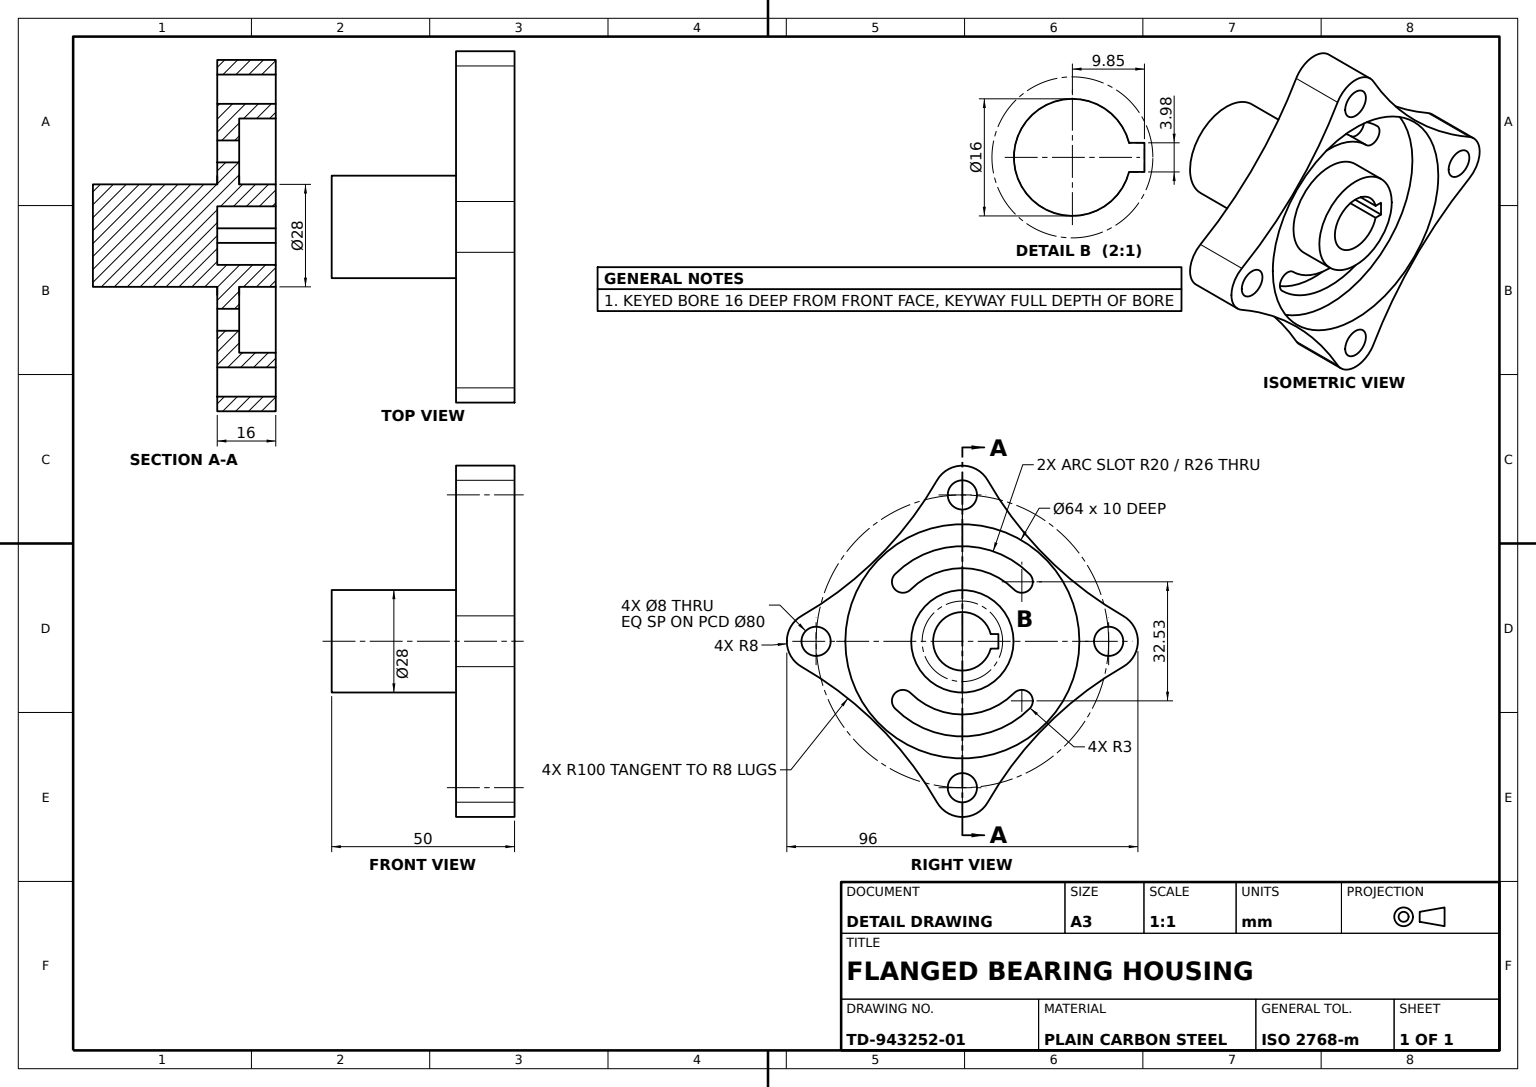
SolidWorks part; units mm, degrees
material "Plain Carbon Steel"
ref_plane "Front Plane" through (0, 0, 0) normal (0, 0, 1) x (1, 0, 0)
ref_plane "Top Plane" through (0, 0, 0) normal (0, 1, 0) x (1, 0, 0)
ref_plane "Right Plane" through (0, 0, 0) normal (1, 0, 0) x (0, 0, -1)
sketch "Flange Plate Sketch" plane through (0, 0, 0) normal (0, 0, 1) x (1, 0, 0)
  line L0 (0, 0) -> (0, 40) construction
  line L1 (0, 0) -> (40, 0) construction
  line L2 (0, 0) -> (0, -40) construction
  line L3 (0, 0) -> (-40, 0) construction
  circle A0 centre (0, 0) radius 40 construction
  circle A1 centre (0, 0) radius 32
  circle A2 centre (0, 40) radius 4
  circle A4 centre (40, 0) radius 4
  circle A5 centre (-40, 0) radius 4
  circle A6 centre (0, -40) radius 4
  arc A7 (6.9409, 43.9779) -> (-6.9409, 43.9779) centre (0, 40) ccw
  arc A8 (-43.9779, 6.9409) -> (-43.9779, -6.9409) centre (-40, 0) ccw
  arc A9 (-6.9409, -43.9779) -> (6.9409, -43.9779) centre (0, -40) ccw
  arc A10 (43.9779, -6.9409) -> (43.9779, 6.9409) centre (40, 0) ccw
  arc A11 (-43.9779, 6.9409) -> (-6.9409, 43.9779) centre (-93.7021, 93.7021) ccw
  arc A12 (6.9409, 43.9779) -> (43.9779, 6.9409) centre (93.7021, 93.7021) ccw
  arc A13 (6.9409, 43.9779) -> (43.9779, 6.9409) centre (93.7021, 93.7021) ccw
  arc A14 (43.9779, -6.9409) -> (6.9409, -43.9779) centre (93.7021, -93.7021) ccw
  arc A15 (-6.9409, -43.9779) -> (-43.9779, -6.9409) centre (-93.7021, -93.7021) ccw
  dimension "D1" = 40
  dimension "D2" = 32
  dimension "D3" = 4
  dimension "D4" = 4
  dimension "D5" = 4
  dimension "D6" = 4
  dimension "D9" = 8
  dimension "D11" = 100
  dimension "D13" = 4
extrude "Flange Plate 4-Lug" add sketch "Flange Plate Sketch" along normal blind 16 contours A15 A9 A14 A10 A12 A7 A11 A8 A6 A5 A4 A2 A1 | A1
sketch "Front Recess Ø32 Sketch" plane through (0, 0, 16) normal (0, 0, 1) x (1, 0, 0)
  circle A0 centre (0, 0) radius 32
  dimension "D1" = 32
extrude "Front Recess Ø32" cut sketch "Front Recess Ø32 Sketch" against normal blind 10
sketch "Arc Slots Sketch" plane through (0, 0, 6) normal (0, 0, 1) x (1, 0, 0)
  arc A0 (-18.3848, -18.3848) -> (18.3848, -18.3848) centre (0, 0) ccw
  arc A1 (-14.1421, -14.1421) -> (14.1421, -14.1421) centre (0, 0) ccw
  arc A2 (14.1421, 14.1421) -> (-14.1421, 14.1421) centre (0, 0) ccw
  arc A3 (18.3848, 18.3848) -> (-18.3848, 18.3848) centre (0, 0) ccw
  arc A4 (-18.3848, 18.3848) -> (-14.1421, 14.1421) centre (-16.2635, 16.2635) ccw
  arc A5 (14.1421, 14.1421) -> (18.3848, 18.3848) centre (16.2635, 16.2635) ccw
  arc A6 (-18.3848, -18.3848) -> (-14.1421, -14.1421) centre (-16.2635, -16.2635) cw
  arc A7 (18.3848, -18.3848) -> (14.1421, -14.1421) centre (16.2635, -16.2635) ccw
  dimension "D3" = 3
  dimension "D4" = 3
  dimension "D7" = 3
  dimension "D8" = 3
  dimension "D1" = 20
  dimension "D2" = 32.5269
extrude "Arc Slots" cut sketch "Arc Slots Sketch" against normal blind 6
sketch "Front Hub Ø14 Sketch" plane through (0, 0, 6) normal (0, 0, 1) x (1, 0, 0)
  circle A0 centre (0, 0) radius 14
  dimension "D1" = 14
extrude "Front Hub Ø14" add sketch "Front Hub Ø14 Sketch" along normal blind 10
sketch "Rear Hub Ø14 Sketch" plane through (0, 0, 0) normal (0, 0, -1) x (-1, 0, 0)
  circle A0 centre (0, 0) radius 14
  dimension "D1" = 14
extrude "Rear Hub Ø14" add sketch "Rear Hub Ø14 Sketch" along normal blind 34
sketch "Keyed Bore Ø8 Sketch" plane through (0, 0, 16) normal (0, 0, 1) x (1, 0, 0)
  line L2 (9.85, 0) -> (9.85, 1.99)
  line L3 (9.85, 1.99) -> (7.7485, 1.99)
  line L5 (7.7485, -1.99) -> (9.85, -1.99)
  line L6 (9.85, -1.99) -> (9.85, 0)
  arc A0 (7.7485, 1.99) -> (7.7485, -1.99) centre (0, 0) ccw
  point P1 (8.7993, -1.99)
  dimension "D1" = 8
  dimension "D2" = 9.85
  dimension "D3" = 1.99
  dimension "D4" = 3.98
  dimension "D5" = 2.1015
extrude "Keyed Bore Ø8" cut sketch "Keyed Bore Ø8 Sketch" against normal blind 16
